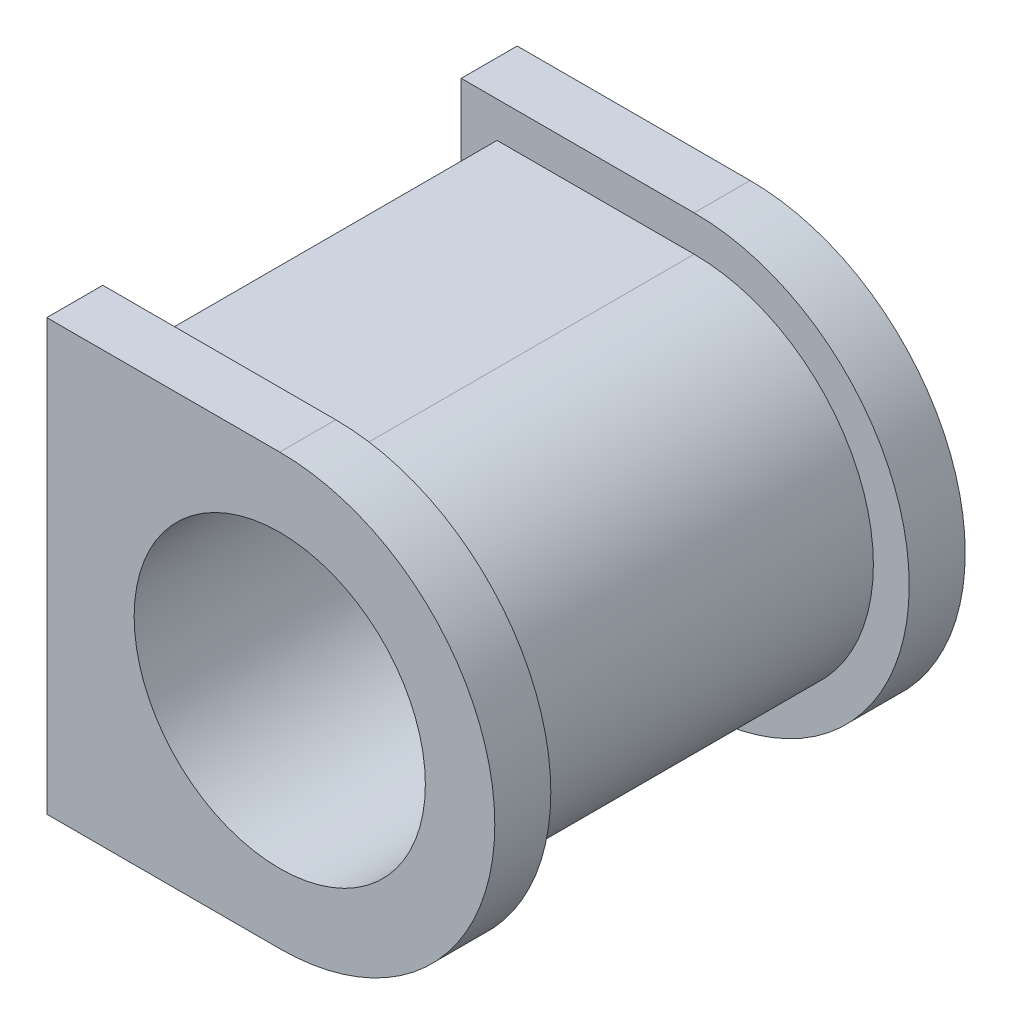
ISO-10303-21;
HEADER;
FILE_DESCRIPTION(('STEP AP214'),'2;1');
FILE_NAME('part.step','',(''),(''),'','','');
FILE_SCHEMA(('AUTOMOTIVE_DESIGN { 1 0 10303 214 1 1 1 1 }'));
ENDSEC;
DATA;
#1=APPLICATION_CONTEXT('core data for automotive mechanical design processes');
#2=APPLICATION_PROTOCOL_DEFINITION('international standard','automotive_design',2000,#1);
#3=PRODUCT_CONTEXT('',#1,'mechanical');
#4=PRODUCT('Part','Part','',(#3));
#5=PRODUCT_RELATED_PRODUCT_CATEGORY('part','',(#4));
#6=PRODUCT_DEFINITION_FORMATION('','',#4);
#7=PRODUCT_DEFINITION_CONTEXT('part definition',#1,'design');
#8=PRODUCT_DEFINITION('design','',#6,#7);
#9=PRODUCT_DEFINITION_SHAPE('','',#8);
#10=(LENGTH_UNIT() NAMED_UNIT(*) SI_UNIT(.MILLI.,.METRE.));
#11=(NAMED_UNIT(*) PLANE_ANGLE_UNIT() SI_UNIT($,.RADIAN.));
#12=(NAMED_UNIT(*) SI_UNIT($,.STERADIAN.) SOLID_ANGLE_UNIT());
#13=UNCERTAINTY_MEASURE_WITH_UNIT(LENGTH_MEASURE(1.E-05),#10,'distance_accuracy_value','');
#14=(GEOMETRIC_REPRESENTATION_CONTEXT(3) GLOBAL_UNCERTAINTY_ASSIGNED_CONTEXT((#13)) GLOBAL_UNIT_ASSIGNED_CONTEXT((#10,
#11,#12)) REPRESENTATION_CONTEXT('',''));
#15=CARTESIAN_POINT('',(0.,0.,0.));
#16=DIRECTION('',(0.,0.,1.));
#17=DIRECTION('',(1.,0.,0.));
#18=AXIS2_PLACEMENT_3D('',#15,#16,#17);
#19=CARTESIAN_POINT('',(0.,0.,40.));
#20=DIRECTION('',(0.,0.,-1.));
#21=DIRECTION('',(-1.,0.,0.));
#22=AXIS2_PLACEMENT_3D('',#19,#20,#21);
#23=CYLINDRICAL_SURFACE('',#22,40.);
#24=CARTESIAN_POINT('',(0.,0.,-40.));
#25=DIRECTION('',(0.,0.,1.));
#26=DIRECTION('',(1.,0.,0.));
#27=AXIS2_PLACEMENT_3D('',#24,#25,#26);
#28=CIRCLE('',#27,40.);
#29=CARTESIAN_POINT('',(0.,-40.,-40.));
#30=VERTEX_POINT('',#29);
#31=CARTESIAN_POINT('',(0.,40.,-40.));
#32=VERTEX_POINT('',#31);
#33=EDGE_CURVE('E203',#30,#32,#28,.T.);
#34=ORIENTED_EDGE('',*,*,#33,.T.);
#35=DIRECTION('',(0.,0.,-1.));
#36=VECTOR('',#35,1.);
#37=CARTESIAN_POINT('',(0.,40.,40.));
#38=LINE('',#37,#36);
#39=CARTESIAN_POINT('',(0.,40.,40.));
#40=VERTEX_POINT('',#39);
#41=EDGE_CURVE('E11',#40,#32,#38,.T.);
#42=ORIENTED_EDGE('',*,*,#41,.F.);
#43=CARTESIAN_POINT('',(0.,0.,40.));
#44=DIRECTION('',(0.,0.,1.));
#45=DIRECTION('',(1.,0.,0.));
#46=AXIS2_PLACEMENT_3D('',#43,#44,#45);
#47=CIRCLE('',#46,40.);
#48=CARTESIAN_POINT('',(0.,-40.,40.));
#49=VERTEX_POINT('',#48);
#50=EDGE_CURVE('E205',#49,#40,#47,.T.);
#51=ORIENTED_EDGE('',*,*,#50,.F.);
#52=DIRECTION('',(0.,0.,-1.));
#53=VECTOR('',#52,1.);
#54=CARTESIAN_POINT('',(0.,-40.,40.));
#55=LINE('',#54,#53);
#56=EDGE_CURVE('E214',#49,#30,#55,.T.);
#57=ORIENTED_EDGE('',*,*,#56,.T.);
#58=EDGE_LOOP('',(#34,#42,#51,#57));
#59=FACE_BOUND('',#58,.T.);
#60=ADVANCED_FACE('F39',(#59),#23,.T.);
#61=CARTESIAN_POINT('',(0.,40.,40.));
#62=DIRECTION('',(0.,-1.,0.));
#63=DIRECTION('',(1.,0.,0.));
#64=AXIS2_PLACEMENT_3D('',#61,#62,#63);
#65=PLANE('',#64);
#66=DIRECTION('',(-1.,0.,0.));
#67=VECTOR('',#66,1.);
#68=CARTESIAN_POINT('',(0.,40.,-40.));
#69=LINE('',#68,#67);
#70=CARTESIAN_POINT('',(-44.,40.,-40.));
#71=VERTEX_POINT('',#70);
#72=EDGE_CURVE('E217',#32,#71,#69,.T.);
#73=ORIENTED_EDGE('',*,*,#72,.T.);
#74=DIRECTION('',(0.,0.,-1.));
#75=VECTOR('',#74,1.);
#76=CARTESIAN_POINT('',(-44.,40.,40.));
#77=LINE('',#76,#75);
#78=CARTESIAN_POINT('',(-44.,40.,40.));
#79=VERTEX_POINT('',#78);
#80=EDGE_CURVE('E50',#79,#71,#77,.T.);
#81=ORIENTED_EDGE('',*,*,#80,.F.);
#82=DIRECTION('',(-1.,0.,0.));
#83=VECTOR('',#82,1.);
#84=CARTESIAN_POINT('',(0.,40.,40.));
#85=LINE('',#84,#83);
#86=EDGE_CURVE('E202',#40,#79,#85,.T.);
#87=ORIENTED_EDGE('',*,*,#86,.F.);
#88=ORIENTED_EDGE('',*,*,#41,.T.);
#89=EDGE_LOOP('',(#73,#81,#87,#88));
#90=FACE_BOUND('',#89,.T.);
#91=ADVANCED_FACE('F234',(#90),#65,.F.);
#92=CARTESIAN_POINT('',(-44.,-40.,40.));
#93=DIRECTION('',(1.,0.,0.));
#94=DIRECTION('',(0.,0.,-1.));
#95=AXIS2_PLACEMENT_3D('',#92,#93,#94);
#96=PLANE('',#95);
#97=DIRECTION('',(0.,-1.,0.));
#98=VECTOR('',#97,1.);
#99=CARTESIAN_POINT('',(-44.,-40.,-40.));
#100=LINE('',#99,#98);
#101=CARTESIAN_POINT('',(-44.,-40.,-40.));
#102=VERTEX_POINT('',#101);
#103=EDGE_CURVE('E222',#71,#102,#100,.T.);
#104=ORIENTED_EDGE('',*,*,#103,.T.);
#105=DIRECTION('',(0.,0.,-1.));
#106=VECTOR('',#105,1.);
#107=CARTESIAN_POINT('',(-44.,-40.,40.));
#108=LINE('',#107,#106);
#109=CARTESIAN_POINT('',(-44.,-40.,40.));
#110=VERTEX_POINT('',#109);
#111=EDGE_CURVE('E53',#110,#102,#108,.T.);
#112=ORIENTED_EDGE('',*,*,#111,.F.);
#113=DIRECTION('',(0.,-1.,0.));
#114=VECTOR('',#113,1.);
#115=CARTESIAN_POINT('',(-44.,-40.,40.));
#116=LINE('',#115,#114);
#117=EDGE_CURVE('E207',#79,#110,#116,.T.);
#118=ORIENTED_EDGE('',*,*,#117,.F.);
#119=ORIENTED_EDGE('',*,*,#80,.T.);
#120=EDGE_LOOP('',(#104,#112,#118,#119));
#121=FACE_BOUND('',#120,.T.);
#122=ADVANCED_FACE('F229',(#121),#96,.F.);
#123=CARTESIAN_POINT('',(0.,-40.,40.));
#124=DIRECTION('',(0.,1.,0.));
#125=DIRECTION('',(-1.,0.,0.));
#126=AXIS2_PLACEMENT_3D('',#123,#124,#125);
#127=PLANE('',#126);
#128=DIRECTION('',(1.,0.,0.));
#129=VECTOR('',#128,1.);
#130=CARTESIAN_POINT('',(0.,-40.,-40.));
#131=LINE('',#130,#129);
#132=EDGE_CURVE('E206',#102,#30,#131,.T.);
#133=ORIENTED_EDGE('',*,*,#132,.T.);
#134=ORIENTED_EDGE('',*,*,#56,.F.);
#135=DIRECTION('',(1.,0.,0.));
#136=VECTOR('',#135,1.);
#137=CARTESIAN_POINT('',(0.,-40.,40.));
#138=LINE('',#137,#136);
#139=EDGE_CURVE('E215',#110,#49,#138,.T.);
#140=ORIENTED_EDGE('',*,*,#139,.F.);
#141=ORIENTED_EDGE('',*,*,#111,.T.);
#142=EDGE_LOOP('',(#133,#134,#140,#141));
#143=FACE_BOUND('',#142,.T.);
#144=ADVANCED_FACE('F236',(#143),#127,.F.);
#145=CARTESIAN_POINT('',(0.,0.,40.));
#146=DIRECTION('',(0.,0.,-1.));
#147=DIRECTION('',(-1.,0.,0.));
#148=AXIS2_PLACEMENT_3D('',#145,#146,#147);
#149=CYLINDRICAL_SURFACE('',#148,32.5);
#150=CARTESIAN_POINT('',(0.,0.,52.5));
#151=DIRECTION('',(0.,0.,1.));
#152=DIRECTION('',(1.,0.,0.));
#153=AXIS2_PLACEMENT_3D('',#150,#151,#152);
#154=CIRCLE('',#153,32.5);
#155=CARTESIAN_POINT('',(32.5,0.,52.5));
#156=VERTEX_POINT('',#155);
#157=EDGE_CURVE('E135',#156,#156,#154,.T.);
#158=ORIENTED_EDGE('',*,*,#157,.T.);
#159=EDGE_LOOP('',(#158));
#160=FACE_BOUND('',#159,.T.);
#161=CARTESIAN_POINT('',(0.,0.,-52.5));
#162=DIRECTION('',(0.,0.,1.));
#163=DIRECTION('',(1.,0.,0.));
#164=AXIS2_PLACEMENT_3D('',#161,#162,#163);
#165=CIRCLE('',#164,32.5);
#166=CARTESIAN_POINT('',(32.5,0.,-52.5));
#167=VERTEX_POINT('',#166);
#168=EDGE_CURVE('E158',#167,#167,#165,.T.);
#169=ORIENTED_EDGE('',*,*,#168,.F.);
#170=EDGE_LOOP('',(#169));
#171=FACE_BOUND('',#170,.T.);
#172=ADVANCED_FACE('F243',(#160,#171),#149,.F.);
#173=CARTESIAN_POINT('',(0.,0.,40.));
#174=DIRECTION('',(0.,0.,1.));
#175=DIRECTION('',(1.,0.,0.));
#176=AXIS2_PLACEMENT_3D('',#173,#174,#175);
#177=PLANE('',#176);
#178=DIRECTION('',(1.,0.,0.));
#179=VECTOR('',#178,1.);
#180=CARTESIAN_POINT('',(-52.,-48.,40.));
#181=LINE('',#180,#179);
#182=CARTESIAN_POINT('',(-52.,-48.,40.));
#183=VERTEX_POINT('',#182);
#184=CARTESIAN_POINT('',(0.,-48.,40.));
#185=VERTEX_POINT('',#184);
#186=EDGE_CURVE('E171',#183,#185,#181,.T.);
#187=ORIENTED_EDGE('',*,*,#186,.F.);
#188=DIRECTION('',(0.,-1.,0.));
#189=VECTOR('',#188,1.);
#190=CARTESIAN_POINT('',(-52.,48.,40.));
#191=LINE('',#190,#189);
#192=CARTESIAN_POINT('',(-52.,48.,40.));
#193=VERTEX_POINT('',#192);
#194=EDGE_CURVE('E179',#193,#183,#191,.T.);
#195=ORIENTED_EDGE('',*,*,#194,.F.);
#196=DIRECTION('',(-1.,0.,0.));
#197=VECTOR('',#196,1.);
#198=CARTESIAN_POINT('',(0.,48.,40.));
#199=LINE('',#198,#197);
#200=CARTESIAN_POINT('',(0.,48.,40.));
#201=VERTEX_POINT('',#200);
#202=EDGE_CURVE('E187',#201,#193,#199,.T.);
#203=ORIENTED_EDGE('',*,*,#202,.F.);
#204=CARTESIAN_POINT('',(0.,0.,40.));
#205=DIRECTION('',(0.,0.,1.));
#206=DIRECTION('',(1.,0.,0.));
#207=AXIS2_PLACEMENT_3D('',#204,#205,#206);
#208=CIRCLE('',#207,48.);
#209=EDGE_CURVE('E183',#185,#201,#208,.T.);
#210=ORIENTED_EDGE('',*,*,#209,.F.);
#211=EDGE_LOOP('',(#187,#195,#203,#210));
#212=FACE_BOUND('',#211,.T.);
#213=ORIENTED_EDGE('',*,*,#139,.T.);
#214=ORIENTED_EDGE('',*,*,#50,.T.);
#215=ORIENTED_EDGE('',*,*,#86,.T.);
#216=ORIENTED_EDGE('',*,*,#117,.T.);
#217=EDGE_LOOP('',(#213,#214,#215,#216));
#218=FACE_BOUND('',#217,.T.);
#219=ADVANCED_FACE('F241',(#212,#218),#177,.F.);
#220=CARTESIAN_POINT('',(0.,0.,52.5));
#221=DIRECTION('',(0.,0.,1.));
#222=DIRECTION('',(1.,0.,0.));
#223=AXIS2_PLACEMENT_3D('',#220,#221,#222);
#224=PLANE('',#223);
#225=DIRECTION('',(1.,0.,0.));
#226=VECTOR('',#225,1.);
#227=CARTESIAN_POINT('',(-52.,-48.,52.5));
#228=LINE('',#227,#226);
#229=CARTESIAN_POINT('',(-52.,-48.,52.5));
#230=VERTEX_POINT('',#229);
#231=CARTESIAN_POINT('',(0.,-48.,52.5));
#232=VERTEX_POINT('',#231);
#233=EDGE_CURVE('E172',#230,#232,#228,.T.);
#234=ORIENTED_EDGE('',*,*,#233,.T.);
#235=CARTESIAN_POINT('',(0.,0.,52.5));
#236=DIRECTION('',(0.,0.,1.));
#237=DIRECTION('',(1.,0.,0.));
#238=AXIS2_PLACEMENT_3D('',#235,#236,#237);
#239=CIRCLE('',#238,48.);
#240=CARTESIAN_POINT('',(0.,48.,52.5));
#241=VERTEX_POINT('',#240);
#242=EDGE_CURVE('E175',#232,#241,#239,.T.);
#243=ORIENTED_EDGE('',*,*,#242,.T.);
#244=DIRECTION('',(-1.,0.,0.));
#245=VECTOR('',#244,1.);
#246=CARTESIAN_POINT('',(0.,48.,52.5));
#247=LINE('',#246,#245);
#248=CARTESIAN_POINT('',(-52.,48.,52.5));
#249=VERTEX_POINT('',#248);
#250=EDGE_CURVE('E180',#241,#249,#247,.T.);
#251=ORIENTED_EDGE('',*,*,#250,.T.);
#252=DIRECTION('',(0.,-1.,0.));
#253=VECTOR('',#252,1.);
#254=CARTESIAN_POINT('',(-52.,48.,52.5));
#255=LINE('',#254,#253);
#256=EDGE_CURVE('E177',#249,#230,#255,.T.);
#257=ORIENTED_EDGE('',*,*,#256,.T.);
#258=EDGE_LOOP('',(#234,#243,#251,#257));
#259=FACE_BOUND('',#258,.T.);
#260=ORIENTED_EDGE('',*,*,#157,.F.);
#261=EDGE_LOOP('',(#260));
#262=FACE_BOUND('',#261,.T.);
#263=ADVANCED_FACE('F244',(#259,#262),#224,.T.);
#264=CARTESIAN_POINT('',(-52.,-48.,52.5));
#265=DIRECTION('',(0.,1.,0.));
#266=DIRECTION('',(-1.,0.,0.));
#267=AXIS2_PLACEMENT_3D('',#264,#265,#266);
#268=PLANE('',#267);
#269=ORIENTED_EDGE('',*,*,#186,.T.);
#270=DIRECTION('',(0.,0.,-1.));
#271=VECTOR('',#270,1.);
#272=CARTESIAN_POINT('',(0.,-48.,52.5));
#273=LINE('',#272,#271);
#274=EDGE_CURVE('E196',#232,#185,#273,.T.);
#275=ORIENTED_EDGE('',*,*,#274,.F.);
#276=ORIENTED_EDGE('',*,*,#233,.F.);
#277=DIRECTION('',(0.,0.,-1.));
#278=VECTOR('',#277,1.);
#279=CARTESIAN_POINT('',(-52.,-48.,52.5));
#280=LINE('',#279,#278);
#281=EDGE_CURVE('E185',#230,#183,#280,.T.);
#282=ORIENTED_EDGE('',*,*,#281,.T.);
#283=EDGE_LOOP('',(#269,#275,#276,#282));
#284=FACE_BOUND('',#283,.T.);
#285=ADVANCED_FACE('F247',(#284),#268,.F.);
#286=CARTESIAN_POINT('',(0.,0.,52.5));
#287=DIRECTION('',(0.,0.,-1.));
#288=DIRECTION('',(-1.,0.,0.));
#289=AXIS2_PLACEMENT_3D('',#286,#287,#288);
#290=CYLINDRICAL_SURFACE('',#289,48.);
#291=ORIENTED_EDGE('',*,*,#209,.T.);
#292=DIRECTION('',(0.,0.,-1.));
#293=VECTOR('',#292,1.);
#294=CARTESIAN_POINT('',(0.,48.,52.5));
#295=LINE('',#294,#293);
#296=EDGE_CURVE('E192',#241,#201,#295,.T.);
#297=ORIENTED_EDGE('',*,*,#296,.F.);
#298=ORIENTED_EDGE('',*,*,#242,.F.);
#299=ORIENTED_EDGE('',*,*,#274,.T.);
#300=EDGE_LOOP('',(#291,#297,#298,#299));
#301=FACE_BOUND('',#300,.T.);
#302=ADVANCED_FACE('F275',(#301),#290,.T.);
#303=CARTESIAN_POINT('',(0.,48.,52.5));
#304=DIRECTION('',(0.,-1.,0.));
#305=DIRECTION('',(1.,0.,0.));
#306=AXIS2_PLACEMENT_3D('',#303,#304,#305);
#307=PLANE('',#306);
#308=ORIENTED_EDGE('',*,*,#202,.T.);
#309=DIRECTION('',(0.,0.,-1.));
#310=VECTOR('',#309,1.);
#311=CARTESIAN_POINT('',(-52.,48.,52.5));
#312=LINE('',#311,#310);
#313=EDGE_CURVE('E191',#249,#193,#312,.T.);
#314=ORIENTED_EDGE('',*,*,#313,.F.);
#315=ORIENTED_EDGE('',*,*,#250,.F.);
#316=ORIENTED_EDGE('',*,*,#296,.T.);
#317=EDGE_LOOP('',(#308,#314,#315,#316));
#318=FACE_BOUND('',#317,.T.);
#319=ADVANCED_FACE('F277',(#318),#307,.F.);
#320=CARTESIAN_POINT('',(-52.,48.,52.5));
#321=DIRECTION('',(1.,0.,0.));
#322=DIRECTION('',(0.,0.,-1.));
#323=AXIS2_PLACEMENT_3D('',#320,#321,#322);
#324=PLANE('',#323);
#325=ORIENTED_EDGE('',*,*,#194,.T.);
#326=ORIENTED_EDGE('',*,*,#281,.F.);
#327=ORIENTED_EDGE('',*,*,#256,.F.);
#328=ORIENTED_EDGE('',*,*,#313,.T.);
#329=EDGE_LOOP('',(#325,#326,#327,#328));
#330=FACE_BOUND('',#329,.T.);
#331=ADVANCED_FACE('F276',(#330),#324,.F.);
#332=CARTESIAN_POINT('',(-52.,-48.,-52.5));
#333=DIRECTION('',(0.,-1.,0.));
#334=DIRECTION('',(1.,0.,0.));
#335=AXIS2_PLACEMENT_3D('',#332,#333,#334);
#336=PLANE('',#335);
#337=DIRECTION('',(1.,0.,0.));
#338=VECTOR('',#337,1.);
#339=CARTESIAN_POINT('',(-52.,-48.,-40.));
#340=LINE('',#339,#338);
#341=CARTESIAN_POINT('',(-52.,-48.,-40.));
#342=VERTEX_POINT('',#341);
#343=CARTESIAN_POINT('',(0.,-48.,-40.));
#344=VERTEX_POINT('',#343);
#345=EDGE_CURVE('E128',#342,#344,#340,.T.);
#346=ORIENTED_EDGE('',*,*,#345,.F.);
#347=DIRECTION('',(0.,0.,1.));
#348=VECTOR('',#347,1.);
#349=CARTESIAN_POINT('',(-52.,-48.,-52.5));
#350=LINE('',#349,#348);
#351=CARTESIAN_POINT('',(-52.,-48.,-52.5));
#352=VERTEX_POINT('',#351);
#353=EDGE_CURVE('E123',#352,#342,#350,.T.);
#354=ORIENTED_EDGE('',*,*,#353,.F.);
#355=DIRECTION('',(1.,0.,0.));
#356=VECTOR('',#355,1.);
#357=CARTESIAN_POINT('',(-52.,-48.,-52.5));
#358=LINE('',#357,#356);
#359=CARTESIAN_POINT('',(0.,-48.,-52.5));
#360=VERTEX_POINT('',#359);
#361=EDGE_CURVE('E130',#352,#360,#358,.T.);
#362=ORIENTED_EDGE('',*,*,#361,.T.);
#363=DIRECTION('',(0.,0.,1.));
#364=VECTOR('',#363,1.);
#365=CARTESIAN_POINT('',(0.,-48.,-52.5));
#366=LINE('',#365,#364);
#367=EDGE_CURVE('E154',#360,#344,#366,.T.);
#368=ORIENTED_EDGE('',*,*,#367,.T.);
#369=EDGE_LOOP('',(#346,#354,#362,#368));
#370=FACE_BOUND('',#369,.T.);
#371=ADVANCED_FACE('F127',(#370),#336,.T.);
#372=CARTESIAN_POINT('',(-52.,48.,-52.5));
#373=DIRECTION('',(-1.,0.,0.));
#374=DIRECTION('',(0.,0.,1.));
#375=AXIS2_PLACEMENT_3D('',#372,#373,#374);
#376=PLANE('',#375);
#377=DIRECTION('',(0.,-1.,0.));
#378=VECTOR('',#377,1.);
#379=CARTESIAN_POINT('',(-52.,48.,-40.));
#380=LINE('',#379,#378);
#381=CARTESIAN_POINT('',(-52.,48.,-40.));
#382=VERTEX_POINT('',#381);
#383=EDGE_CURVE('E160',#382,#342,#380,.T.);
#384=ORIENTED_EDGE('',*,*,#383,.F.);
#385=DIRECTION('',(0.,0.,1.));
#386=VECTOR('',#385,1.);
#387=CARTESIAN_POINT('',(-52.,48.,-52.5));
#388=LINE('',#387,#386);
#389=CARTESIAN_POINT('',(-52.,48.,-52.5));
#390=VERTEX_POINT('',#389);
#391=EDGE_CURVE('E139',#390,#382,#388,.T.);
#392=ORIENTED_EDGE('',*,*,#391,.F.);
#393=DIRECTION('',(0.,-1.,0.));
#394=VECTOR('',#393,1.);
#395=CARTESIAN_POINT('',(-52.,48.,-52.5));
#396=LINE('',#395,#394);
#397=EDGE_CURVE('E142',#390,#352,#396,.T.);
#398=ORIENTED_EDGE('',*,*,#397,.T.);
#399=ORIENTED_EDGE('',*,*,#353,.T.);
#400=EDGE_LOOP('',(#384,#392,#398,#399));
#401=FACE_BOUND('',#400,.T.);
#402=ADVANCED_FACE('F146',(#401),#376,.T.);
#403=CARTESIAN_POINT('',(0.,48.,-52.5));
#404=DIRECTION('',(0.,1.,0.));
#405=DIRECTION('',(-1.,0.,0.));
#406=AXIS2_PLACEMENT_3D('',#403,#404,#405);
#407=PLANE('',#406);
#408=DIRECTION('',(-1.,0.,0.));
#409=VECTOR('',#408,1.);
#410=CARTESIAN_POINT('',(0.,48.,-40.));
#411=LINE('',#410,#409);
#412=CARTESIAN_POINT('',(0.,48.,-40.));
#413=VERTEX_POINT('',#412);
#414=EDGE_CURVE('E159',#413,#382,#411,.T.);
#415=ORIENTED_EDGE('',*,*,#414,.F.);
#416=DIRECTION('',(0.,0.,1.));
#417=VECTOR('',#416,1.);
#418=CARTESIAN_POINT('',(0.,48.,-52.5));
#419=LINE('',#418,#417);
#420=CARTESIAN_POINT('',(0.,48.,-52.5));
#421=VERTEX_POINT('',#420);
#422=EDGE_CURVE('E167',#421,#413,#419,.T.);
#423=ORIENTED_EDGE('',*,*,#422,.F.);
#424=DIRECTION('',(-1.,0.,0.));
#425=VECTOR('',#424,1.);
#426=CARTESIAN_POINT('',(0.,48.,-52.5));
#427=LINE('',#426,#425);
#428=EDGE_CURVE('E149',#421,#390,#427,.T.);
#429=ORIENTED_EDGE('',*,*,#428,.T.);
#430=ORIENTED_EDGE('',*,*,#391,.T.);
#431=EDGE_LOOP('',(#415,#423,#429,#430));
#432=FACE_BOUND('',#431,.T.);
#433=ADVANCED_FACE('F310',(#432),#407,.T.);
#434=CARTESIAN_POINT('',(0.,0.,-52.5));
#435=DIRECTION('',(0.,0.,1.));
#436=DIRECTION('',(1.,0.,0.));
#437=AXIS2_PLACEMENT_3D('',#434,#435,#436);
#438=CYLINDRICAL_SURFACE('',#437,48.);
#439=CARTESIAN_POINT('',(0.,0.,-40.));
#440=DIRECTION('',(0.,0.,1.));
#441=DIRECTION('',(1.,0.,0.));
#442=AXIS2_PLACEMENT_3D('',#439,#440,#441);
#443=CIRCLE('',#442,48.);
#444=EDGE_CURVE('E148',#344,#413,#443,.T.);
#445=ORIENTED_EDGE('',*,*,#444,.F.);
#446=ORIENTED_EDGE('',*,*,#367,.F.);
#447=CARTESIAN_POINT('',(0.,0.,-52.5));
#448=DIRECTION('',(0.,0.,1.));
#449=DIRECTION('',(1.,0.,0.));
#450=AXIS2_PLACEMENT_3D('',#447,#448,#449);
#451=CIRCLE('',#450,48.);
#452=EDGE_CURVE('E144',#360,#421,#451,.T.);
#453=ORIENTED_EDGE('',*,*,#452,.T.);
#454=ORIENTED_EDGE('',*,*,#422,.T.);
#455=EDGE_LOOP('',(#445,#446,#453,#454));
#456=FACE_BOUND('',#455,.T.);
#457=ADVANCED_FACE('F301',(#456),#438,.T.);
#458=CARTESIAN_POINT('',(0.,0.,-52.5));
#459=DIRECTION('',(0.,0.,-1.));
#460=DIRECTION('',(1.,0.,0.));
#461=AXIS2_PLACEMENT_3D('',#458,#459,#460);
#462=PLANE('',#461);
#463=ORIENTED_EDGE('',*,*,#168,.T.);
#464=EDGE_LOOP('',(#463));
#465=FACE_BOUND('',#464,.T.);
#466=ORIENTED_EDGE('',*,*,#361,.F.);
#467=ORIENTED_EDGE('',*,*,#397,.F.);
#468=ORIENTED_EDGE('',*,*,#428,.F.);
#469=ORIENTED_EDGE('',*,*,#452,.F.);
#470=EDGE_LOOP('',(#466,#467,#468,#469));
#471=FACE_BOUND('',#470,.T.);
#472=ADVANCED_FACE('F137',(#465,#471),#462,.T.);
#473=CARTESIAN_POINT('',(0.,0.,-40.));
#474=DIRECTION('',(0.,0.,-1.));
#475=DIRECTION('',(1.,0.,0.));
#476=AXIS2_PLACEMENT_3D('',#473,#474,#475);
#477=PLANE('',#476);
#478=ORIENTED_EDGE('',*,*,#33,.F.);
#479=ORIENTED_EDGE('',*,*,#132,.F.);
#480=ORIENTED_EDGE('',*,*,#103,.F.);
#481=ORIENTED_EDGE('',*,*,#72,.F.);
#482=EDGE_LOOP('',(#478,#479,#480,#481));
#483=FACE_BOUND('',#482,.T.);
#484=ORIENTED_EDGE('',*,*,#345,.T.);
#485=ORIENTED_EDGE('',*,*,#444,.T.);
#486=ORIENTED_EDGE('',*,*,#414,.T.);
#487=ORIENTED_EDGE('',*,*,#383,.T.);
#488=EDGE_LOOP('',(#484,#485,#486,#487));
#489=FACE_BOUND('',#488,.T.);
#490=ADVANCED_FACE('F233',(#483,#489),#477,.F.);
#491=CLOSED_SHELL('',(#60,#91,#122,#144,#172,#219,#263,#285,#302,#319,#331,#371,#402,#433,#457,
#472,#490));
#492=MANIFOLD_SOLID_BREP('B2',#491);
#493=ADVANCED_BREP_SHAPE_REPRESENTATION('',(#18,#492),#14);
#494=SHAPE_DEFINITION_REPRESENTATION(#9,#493);
ENDSEC;
END-ISO-10303-21;
